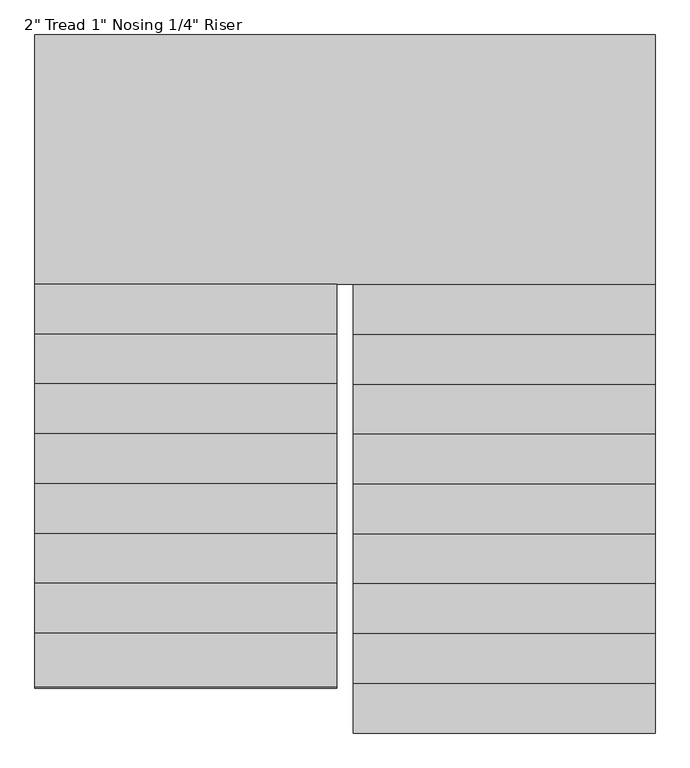
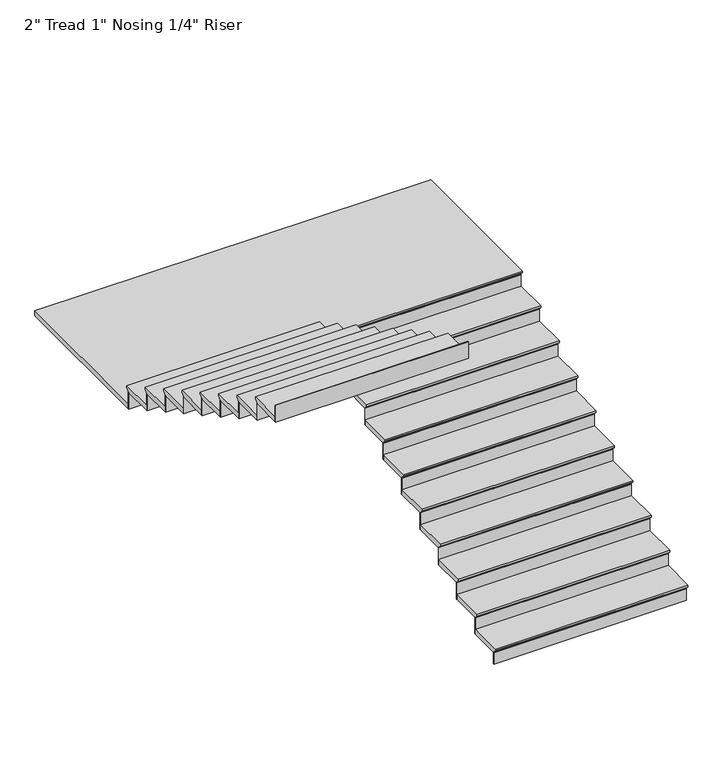
"""IFC4 building model written with IfcOpenShell, lengths in millimetres: stair flight geometry."""

from ifc_helpers import new_model, si_unit, origin, place, context, project, spatial, faceted_brep, source, transform, mapped, element, save


def stair_flight_059c6031(model_context):
    return source(origin(), model_context, "Body", "Brep", [
        faceted_brep([(7785.2813124, -8648.1976656, 4111.7921053), (7785.2813124, -8648.1976656, 4130.8421053), (5940.6255016, -8648.1976656, 4130.8421053), (5940.6255016, -8648.1976656, 4111.7921053), (7785.2813124, -8622.7976656, 4086.3921053), (5940.6255016, -8622.7976656, 4086.3921053), (7785.2813124, -8317.9976656, 4130.8421053), (5940.6255016, -8317.9976656, 4130.8421053), (5940.6255016, -8622.7976656, 4080.0421053), (5940.6255016, -8317.9976656, 4080.0421053), (7785.2813124, -8317.9976656, 4080.0421053), (7785.2813124, -8622.7976656, 4080.0421053)], [[[0, 1, 2, 3]], [[4, 0, 3, 5]], [[2, 1, 6, 7]], [[8, 9, 10, 11]], [[2, 7, 9, 8, 5, 3]], [[8, 11, 4, 5]], [[6, 1, 0, 4, 11, 10]], [[7, 6, 10, 9]]]),
        faceted_brep([(7785.2813124, -8622.7976656, 4080.0421053), (7785.2813124, -8622.7976656, 3962.4), (7785.2813124, -8616.4476656, 3962.4), (7785.2813124, -8616.4476656, 4080.0421053), (5940.6255016, -8622.7976656, 4080.0421053), (5940.6255016, -8616.4476656, 4080.0421053), (5940.6255016, -8616.4476656, 3962.4), (5940.6255016, -8622.7976656, 3962.4)], [[[0, 1, 2, 3]], [[4, 5, 6, 7]], [[1, 0, 4, 7]], [[2, 1, 7, 6]], [[3, 2, 6, 5]], [[0, 3, 5, 4]]]),
        faceted_brep([(7785.2813124, -8317.9976656, 4248.4842105), (7785.2813124, -8317.9976656, 4080.0421053), (7785.2813124, -8311.6476656, 4080.0421053), (7785.2813124, -8311.6476656, 4248.4842105), (5940.6255016, -8317.9976656, 4248.4842105), (5940.6255016, -8311.6476656, 4248.4842105), (5940.6255016, -8311.6476656, 4080.0421053), (5940.6255016, -8317.9976656, 4080.0421053)], [[[0, 1, 2, 3]], [[4, 5, 6, 7]], [[1, 0, 4, 7]], [[2, 1, 7, 6]], [[3, 2, 6, 5]], [[0, 3, 5, 4]]]),
        faceted_brep([(5940.6255016, -8343.3976656, 4299.2842105), (7785.2813124, -8343.3976656, 4299.2842105), (7785.2813124, -8013.1976656, 4299.2842105), (5940.6255016, -8013.1976656, 4299.2842105), (5940.6255016, -8317.9976656, 4248.4842105), (5940.6255016, -8013.1976656, 4248.4842105), (7785.2813124, -8013.1976656, 4248.4842105), (7785.2813124, -8317.9976656, 4248.4842105), (5940.6255016, -8317.9976656, 4254.8342105), (5940.6255016, -8343.3976656, 4280.2342105), (7785.2813124, -8317.9976656, 4254.8342105), (7785.2813124, -8343.3976656, 4280.2342105)], [[[0, 1, 2, 3]], [[4, 5, 6, 7]], [[0, 3, 5, 4, 8, 9]], [[4, 7, 10, 8]], [[2, 1, 11, 10, 7, 6]], [[3, 2, 6, 5]], [[11, 1, 0, 9]], [[10, 11, 9, 8]]]),
        faceted_brep([(7785.2813124, -8013.1976656, 4416.9263158), (7785.2813124, -8013.1976656, 4248.4842105), (7785.2813124, -8006.8476656, 4248.4842105), (7785.2813124, -8006.8476656, 4416.9263158), (5940.6255016, -8013.1976656, 4416.9263158), (5940.6255016, -8006.8476656, 4416.9263158), (5940.6255016, -8006.8476656, 4248.4842105), (5940.6255016, -8013.1976656, 4248.4842105)], [[[0, 1, 2, 3]], [[4, 5, 6, 7]], [[1, 0, 4, 7]], [[2, 1, 7, 6]], [[3, 2, 6, 5]], [[0, 3, 5, 4]]]),
        faceted_brep([(5940.6255016, -8038.5976656, 4467.7263158), (7785.2813124, -8038.5976656, 4467.7263158), (7785.2813124, -7708.3976656, 4467.7263158), (5940.6255016, -7708.3976656, 4467.7263158), (5940.6255016, -8013.1976656, 4416.9263158), (5940.6255016, -7708.3976656, 4416.9263158), (7785.2813124, -7708.3976656, 4416.9263158), (7785.2813124, -8013.1976656, 4416.9263158), (5940.6255016, -8013.1976656, 4423.2763158), (5940.6255016, -8038.5976656, 4448.6763158), (7785.2813124, -8013.1976656, 4423.2763158), (7785.2813124, -8038.5976656, 4448.6763158)], [[[0, 1, 2, 3]], [[4, 5, 6, 7]], [[0, 3, 5, 4, 8, 9]], [[4, 7, 10, 8]], [[2, 1, 11, 10, 7, 6]], [[3, 2, 6, 5]], [[11, 1, 0, 9]], [[10, 11, 9, 8]]]),
        faceted_brep([(7785.2813124, -7708.3976656, 4585.3684211), (7785.2813124, -7708.3976656, 4416.9263158), (7785.2813124, -7702.0476656, 4416.9263158), (7785.2813124, -7702.0476656, 4585.3684211), (5940.6255016, -7708.3976656, 4585.3684211), (5940.6255016, -7702.0476656, 4585.3684211), (5940.6255016, -7702.0476656, 4416.9263158), (5940.6255016, -7708.3976656, 4416.9263158)], [[[0, 1, 2, 3]], [[4, 5, 6, 7]], [[1, 0, 4, 7]], [[2, 1, 7, 6]], [[3, 2, 6, 5]], [[0, 3, 5, 4]]]),
        faceted_brep([(5940.6255016, -7733.7976656, 4636.1684211), (7785.2813124, -7733.7976656, 4636.1684211), (7785.2813124, -7403.5976656, 4636.1684211), (5940.6255016, -7403.5976656, 4636.1684211), (5940.6255016, -7708.3976656, 4585.3684211), (5940.6255016, -7403.5976656, 4585.3684211), (7785.2813124, -7403.5976656, 4585.3684211), (7785.2813124, -7708.3976656, 4585.3684211), (5940.6255016, -7708.3976656, 4591.7184211), (5940.6255016, -7733.7976656, 4617.1184211), (7785.2813124, -7708.3976656, 4591.7184211), (7785.2813124, -7733.7976656, 4617.1184211)], [[[0, 1, 2, 3]], [[4, 5, 6, 7]], [[0, 3, 5, 4, 8, 9]], [[4, 7, 10, 8]], [[2, 1, 11, 10, 7, 6]], [[3, 2, 6, 5]], [[11, 1, 0, 9]], [[10, 11, 9, 8]]]),
        faceted_brep([(7785.2813124, -7403.5976656, 4753.8105263), (7785.2813124, -7403.5976656, 4585.3684211), (7785.2813124, -7397.2476656, 4585.3684211), (7785.2813124, -7397.2476656, 4753.8105263), (5940.6255016, -7403.5976656, 4753.8105263), (5940.6255016, -7397.2476656, 4753.8105263), (5940.6255016, -7397.2476656, 4585.3684211), (5940.6255016, -7403.5976656, 4585.3684211)], [[[0, 1, 2, 3]], [[4, 5, 6, 7]], [[1, 0, 4, 7]], [[2, 1, 7, 6]], [[3, 2, 6, 5]], [[0, 3, 5, 4]]]),
        faceted_brep([(5940.6255016, -7428.9976656, 4804.6105263), (7785.2813124, -7428.9976656, 4804.6105263), (7785.2813124, -7098.7976656, 4804.6105263), (5940.6255016, -7098.7976656, 4804.6105263), (5940.6255016, -7403.5976656, 4753.8105263), (5940.6255016, -7098.7976656, 4753.8105263), (7785.2813124, -7098.7976656, 4753.8105263), (7785.2813124, -7403.5976656, 4753.8105263), (5940.6255016, -7403.5976656, 4760.1605263), (5940.6255016, -7428.9976656, 4785.5605263), (7785.2813124, -7403.5976656, 4760.1605263), (7785.2813124, -7428.9976656, 4785.5605263)], [[[0, 1, 2, 3]], [[4, 5, 6, 7]], [[0, 3, 5, 4, 8, 9]], [[4, 7, 10, 8]], [[2, 1, 11, 10, 7, 6]], [[3, 2, 6, 5]], [[11, 1, 0, 9]], [[10, 11, 9, 8]]]),
        faceted_brep([(7785.2813124, -7098.7976656, 4922.2526316), (7785.2813124, -7098.7976656, 4753.8105263), (7785.2813124, -7092.4476656, 4753.8105263), (7785.2813124, -7092.4476656, 4922.2526316), (5940.6255016, -7098.7976656, 4922.2526316), (5940.6255016, -7092.4476656, 4922.2526316), (5940.6255016, -7092.4476656, 4753.8105263), (5940.6255016, -7098.7976656, 4753.8105263)], [[[0, 1, 2, 3]], [[4, 5, 6, 7]], [[1, 0, 4, 7]], [[2, 1, 7, 6]], [[3, 2, 6, 5]], [[0, 3, 5, 4]]]),
        faceted_brep([(5940.6255016, -7124.1976656, 4973.0526316), (7785.2813124, -7124.1976656, 4973.0526316), (7785.2813124, -6793.9976656, 4973.0526316), (5940.6255016, -6793.9976656, 4973.0526316), (5940.6255016, -7098.7976656, 4922.2526316), (5940.6255016, -6793.9976656, 4922.2526316), (7785.2813124, -6793.9976656, 4922.2526316), (7785.2813124, -7098.7976656, 4922.2526316), (5940.6255016, -7098.7976656, 4928.6026316), (5940.6255016, -7124.1976656, 4954.0026316), (7785.2813124, -7098.7976656, 4928.6026316), (7785.2813124, -7124.1976656, 4954.0026316)], [[[0, 1, 2, 3]], [[4, 5, 6, 7]], [[0, 3, 5, 4, 8, 9]], [[4, 7, 10, 8]], [[2, 1, 11, 10, 7, 6]], [[3, 2, 6, 5]], [[11, 1, 0, 9]], [[10, 11, 9, 8]]]),
        faceted_brep([(7785.2813124, -6793.9976656, 5090.6947368), (7785.2813124, -6793.9976656, 4922.2526316), (7785.2813124, -6787.6476656, 4922.2526316), (7785.2813124, -6787.6476656, 5090.6947368), (5940.6255016, -6793.9976656, 5090.6947368), (5940.6255016, -6787.6476656, 5090.6947368), (5940.6255016, -6787.6476656, 4922.2526316), (5940.6255016, -6793.9976656, 4922.2526316)], [[[0, 1, 2, 3]], [[4, 5, 6, 7]], [[1, 0, 4, 7]], [[2, 1, 7, 6]], [[3, 2, 6, 5]], [[0, 3, 5, 4]]]),
        faceted_brep([(5940.6255016, -6819.3976656, 5141.4947368), (7785.2813124, -6819.3976656, 5141.4947368), (7785.2813124, -6489.1976656, 5141.4947368), (5940.6255016, -6489.1976656, 5141.4947368), (5940.6255016, -6793.9976656, 5090.6947368), (5940.6255016, -6489.1976656, 5090.6947368), (7785.2813124, -6489.1976656, 5090.6947368), (7785.2813124, -6793.9976656, 5090.6947368), (5940.6255016, -6793.9976656, 5097.0447368), (5940.6255016, -6819.3976656, 5122.4447368), (7785.2813124, -6793.9976656, 5097.0447368), (7785.2813124, -6819.3976656, 5122.4447368)], [[[0, 1, 2, 3]], [[4, 5, 6, 7]], [[0, 3, 5, 4, 8, 9]], [[4, 7, 10, 8]], [[2, 1, 11, 10, 7, 6]], [[3, 2, 6, 5]], [[11, 1, 0, 9]], [[10, 11, 9, 8]]]),
        faceted_brep([(7785.2813124, -6489.1976656, 5259.1368421), (7785.2813124, -6489.1976656, 5090.6947368), (7785.2813124, -6482.8476656, 5090.6947368), (7785.2813124, -6482.8476656, 5259.1368421), (5940.6255016, -6489.1976656, 5259.1368421), (5940.6255016, -6482.8476656, 5259.1368421), (5940.6255016, -6482.8476656, 5090.6947368), (5940.6255016, -6489.1976656, 5090.6947368)], [[[0, 1, 2, 3]], [[4, 5, 6, 7]], [[1, 0, 4, 7]], [[2, 1, 7, 6]], [[3, 2, 6, 5]], [[0, 3, 5, 4]]]),
        faceted_brep([(5940.6255016, -6514.5976656, 5309.9368421), (7785.2813124, -6514.5976656, 5309.9368421), (7785.2813124, -6184.3976656, 5309.9368421), (5940.6255016, -6184.3976656, 5309.9368421), (5940.6255016, -6489.1976656, 5259.1368421), (5940.6255016, -6184.3976656, 5259.1368421), (7785.2813124, -6184.3976656, 5259.1368421), (7785.2813124, -6489.1976656, 5259.1368421), (5940.6255016, -6489.1976656, 5265.4868421), (5940.6255016, -6514.5976656, 5290.8868421), (7785.2813124, -6489.1976656, 5265.4868421), (7785.2813124, -6514.5976656, 5290.8868421)], [[[0, 1, 2, 3]], [[4, 5, 6, 7]], [[0, 3, 5, 4, 8, 9]], [[4, 7, 10, 8]], [[2, 1, 11, 10, 7, 6]], [[3, 2, 6, 5]], [[11, 1, 0, 9]], [[10, 11, 9, 8]]]),
        faceted_brep([(7785.2813124, -5879.5976656, 5596.0210526), (7785.2813124, -5879.5976656, 5427.5789474), (7785.2813124, -5873.2476656, 5427.5789474), (7785.2813124, -5873.2476656, 5596.0210526), (5940.6255016, -5879.5976656, 5596.0210526), (5940.6255016, -5873.2476656, 5596.0210526), (5940.6255016, -5873.2476656, 5427.5789474), (5940.6255016, -5879.5976656, 5427.5789474)], [[[0, 1, 2, 3]], [[4, 5, 6, 7]], [[1, 0, 4, 7]], [[2, 1, 7, 6]], [[3, 2, 6, 5]], [[0, 3, 5, 4]]]),
        faceted_brep([(5839.0255016, -5930.3976656, 5646.8210526), (5839.0255016, -5904.9976656, 5646.8210526), (7785.2813124, -5904.9976656, 5646.8210526), (7785.2813124, -4380.9976656, 5646.8210526), (3994.3696908, -4380.9976656, 5646.8210526), (3994.3696908, -5930.3976656, 5646.8210526), (5839.0255016, -5904.9976656, 5596.0210526), (5839.0255016, -5930.3976656, 5596.0210526), (3994.3696908, -5930.3976656, 5596.0210526), (3994.3696908, -4380.9976656, 5596.0210526), (7785.2813124, -4380.9976656, 5596.0210526), (7785.2813124, -5879.5976656, 5596.0210526), (5940.6255016, -5879.5976656, 5596.0210526), (5940.6255016, -5904.9976656, 5596.0210526), (7785.2813124, -5879.5976656, 5602.3710526), (5940.6255016, -5879.5976656, 5602.3710526), (7785.2813124, -5904.9976656, 5627.7710526), (5940.6255016, -5904.9976656, 5627.7710526)], [[[0, 1, 2, 3, 4, 5]], [[6, 7, 8, 9, 10, 11, 12, 13]], [[1, 0, 7, 6]], [[12, 11, 14, 15]], [[3, 2, 16, 14, 11, 10]], [[0, 5, 8, 7]], [[14, 16, 17, 15]], [[2, 1, 6, 13, 17, 16]], [[13, 12, 15, 17]], [[4, 3, 10, 9]], [[5, 4, 9, 8]]]),
        faceted_brep([(3994.3696908, -8368.7976656, 7112.0), (3994.3696908, -8368.7976656, 6943.5578947), (3994.3696908, -8375.1476656, 6943.5578947), (3994.3696908, -8375.1476656, 7112.0), (5839.0255016, -8368.7976656, 7112.0), (5839.0255016, -8375.1476656, 7112.0), (5839.0255016, -8375.1476656, 6943.5578947), (5839.0255016, -8368.7976656, 6943.5578947)], [[[0, 1, 2, 3]], [[4, 5, 6, 7]], [[1, 0, 4, 7]], [[2, 1, 7, 6]], [[3, 2, 6, 5]], [[0, 3, 5, 4]]]),
        faceted_brep([(7785.2813124, -6184.3976656, 5427.5789474), (7785.2813124, -6184.3976656, 5259.1368421), (7785.2813124, -6178.0476656, 5259.1368421), (7785.2813124, -6178.0476656, 5427.5789474), (5940.6255016, -6184.3976656, 5427.5789474), (5940.6255016, -6178.0476656, 5427.5789474), (5940.6255016, -6178.0476656, 5259.1368421), (5940.6255016, -6184.3976656, 5259.1368421)], [[[0, 1, 2, 3]], [[4, 5, 6, 7]], [[1, 0, 4, 7]], [[2, 1, 7, 6]], [[3, 2, 6, 5]], [[0, 3, 5, 4]]]),
        faceted_brep([(5940.6255016, -6209.7976656, 5478.3789474), (7785.2813124, -6209.7976656, 5478.3789474), (7785.2813124, -5879.5976656, 5478.3789474), (5940.6255016, -5879.5976656, 5478.3789474), (5940.6255016, -6184.3976656, 5427.5789474), (5940.6255016, -5879.5976656, 5427.5789474), (7785.2813124, -5879.5976656, 5427.5789474), (7785.2813124, -6184.3976656, 5427.5789474), (5940.6255016, -6184.3976656, 5433.9289474), (5940.6255016, -6209.7976656, 5459.3289474), (7785.2813124, -6184.3976656, 5433.9289474), (7785.2813124, -6209.7976656, 5459.3289474)], [[[0, 1, 2, 3]], [[4, 5, 6, 7]], [[0, 3, 5, 4, 8, 9]], [[4, 7, 10, 8]], [[2, 1, 11, 10, 7, 6]], [[3, 2, 6, 5]], [[11, 1, 0, 9]], [[10, 11, 9, 8]]]),
        faceted_brep([(3994.3696908, -5930.3976656, 5764.4631579), (3994.3696908, -5930.3976656, 5596.0210526), (3994.3696908, -5936.7476656, 5596.0210526), (3994.3696908, -5936.7476656, 5764.4631579), (5839.0255016, -5930.3976656, 5764.4631579), (5839.0255016, -5936.7476656, 5764.4631579), (5839.0255016, -5936.7476656, 5596.0210526), (5839.0255016, -5930.3976656, 5596.0210526)], [[[0, 1, 2, 3]], [[4, 5, 6, 7]], [[1, 0, 4, 7]], [[2, 1, 7, 6]], [[3, 2, 6, 5]], [[0, 3, 5, 4]]]),
        faceted_brep([(5839.0255016, -5904.9976656, 5815.2631579), (3994.3696908, -5904.9976656, 5815.2631579), (3994.3696908, -6235.1976656, 5815.2631579), (5839.0255016, -6235.1976656, 5815.2631579), (5839.0255016, -5930.3976656, 5764.4631579), (5839.0255016, -6235.1976656, 5764.4631579), (3994.3696908, -6235.1976656, 5764.4631579), (3994.3696908, -5930.3976656, 5764.4631579), (5839.0255016, -5930.3976656, 5770.8131579), (5839.0255016, -5904.9976656, 5796.2131579), (3994.3696908, -5930.3976656, 5770.8131579), (3994.3696908, -5904.9976656, 5796.2131579)], [[[0, 1, 2, 3]], [[4, 5, 6, 7]], [[0, 3, 5, 4, 8, 9]], [[4, 7, 10, 8]], [[2, 1, 11, 10, 7, 6]], [[3, 2, 6, 5]], [[11, 1, 0, 9]], [[10, 11, 9, 8]]]),
        faceted_brep([(3994.3696908, -6235.1976656, 5932.9052632), (3994.3696908, -6235.1976656, 5764.4631579), (3994.3696908, -6241.5476656, 5764.4631579), (3994.3696908, -6241.5476656, 5932.9052632), (5839.0255016, -6235.1976656, 5932.9052632), (5839.0255016, -6241.5476656, 5932.9052632), (5839.0255016, -6241.5476656, 5764.4631579), (5839.0255016, -6235.1976656, 5764.4631579)], [[[0, 1, 2, 3]], [[4, 5, 6, 7]], [[1, 0, 4, 7]], [[2, 1, 7, 6]], [[3, 2, 6, 5]], [[0, 3, 5, 4]]]),
        faceted_brep([(5839.0255016, -6209.7976656, 5983.7052632), (3994.3696908, -6209.7976656, 5983.7052632), (3994.3696908, -6539.9976656, 5983.7052632), (5839.0255016, -6539.9976656, 5983.7052632), (5839.0255016, -6235.1976656, 5932.9052632), (5839.0255016, -6539.9976656, 5932.9052632), (3994.3696908, -6539.9976656, 5932.9052632), (3994.3696908, -6235.1976656, 5932.9052632), (5839.0255016, -6235.1976656, 5939.2552632), (5839.0255016, -6209.7976656, 5964.6552632), (3994.3696908, -6235.1976656, 5939.2552632), (3994.3696908, -6209.7976656, 5964.6552632)], [[[0, 1, 2, 3]], [[4, 5, 6, 7]], [[0, 3, 5, 4, 8, 9]], [[4, 7, 10, 8]], [[2, 1, 11, 10, 7, 6]], [[3, 2, 6, 5]], [[11, 1, 0, 9]], [[10, 11, 9, 8]]]),
        faceted_brep([(3994.3696908, -6539.9976656, 6101.3473684), (3994.3696908, -6539.9976656, 5932.9052632), (3994.3696908, -6546.3476656, 5932.9052632), (3994.3696908, -6546.3476656, 6101.3473684), (5839.0255016, -6539.9976656, 6101.3473684), (5839.0255016, -6546.3476656, 6101.3473684), (5839.0255016, -6546.3476656, 5932.9052632), (5839.0255016, -6539.9976656, 5932.9052632)], [[[0, 1, 2, 3]], [[4, 5, 6, 7]], [[1, 0, 4, 7]], [[2, 1, 7, 6]], [[3, 2, 6, 5]], [[0, 3, 5, 4]]]),
        faceted_brep([(5839.0255016, -6514.5976656, 6152.1473684), (3994.3696908, -6514.5976656, 6152.1473684), (3994.3696908, -6844.7976656, 6152.1473684), (5839.0255016, -6844.7976656, 6152.1473684), (5839.0255016, -6539.9976656, 6101.3473684), (5839.0255016, -6844.7976656, 6101.3473684), (3994.3696908, -6844.7976656, 6101.3473684), (3994.3696908, -6539.9976656, 6101.3473684), (5839.0255016, -6539.9976656, 6107.6973684), (5839.0255016, -6514.5976656, 6133.0973684), (3994.3696908, -6539.9976656, 6107.6973684), (3994.3696908, -6514.5976656, 6133.0973684)], [[[0, 1, 2, 3]], [[4, 5, 6, 7]], [[0, 3, 5, 4, 8, 9]], [[4, 7, 10, 8]], [[2, 1, 11, 10, 7, 6]], [[3, 2, 6, 5]], [[11, 1, 0, 9]], [[10, 11, 9, 8]]]),
        faceted_brep([(3994.3696908, -6844.7976656, 6269.7894737), (3994.3696908, -6844.7976656, 6101.3473684), (3994.3696908, -6851.1476656, 6101.3473684), (3994.3696908, -6851.1476656, 6269.7894737), (5839.0255016, -6844.7976656, 6269.7894737), (5839.0255016, -6851.1476656, 6269.7894737), (5839.0255016, -6851.1476656, 6101.3473684), (5839.0255016, -6844.7976656, 6101.3473684)], [[[0, 1, 2, 3]], [[4, 5, 6, 7]], [[1, 0, 4, 7]], [[2, 1, 7, 6]], [[3, 2, 6, 5]], [[0, 3, 5, 4]]]),
        faceted_brep([(5839.0255016, -6819.3976656, 6320.5894737), (3994.3696908, -6819.3976656, 6320.5894737), (3994.3696908, -7149.5976656, 6320.5894737), (5839.0255016, -7149.5976656, 6320.5894737), (5839.0255016, -6844.7976656, 6269.7894737), (5839.0255016, -7149.5976656, 6269.7894737), (3994.3696908, -7149.5976656, 6269.7894737), (3994.3696908, -6844.7976656, 6269.7894737), (5839.0255016, -6844.7976656, 6276.1394737), (5839.0255016, -6819.3976656, 6301.5394737), (3994.3696908, -6844.7976656, 6276.1394737), (3994.3696908, -6819.3976656, 6301.5394737)], [[[0, 1, 2, 3]], [[4, 5, 6, 7]], [[0, 3, 5, 4, 8, 9]], [[4, 7, 10, 8]], [[2, 1, 11, 10, 7, 6]], [[3, 2, 6, 5]], [[11, 1, 0, 9]], [[10, 11, 9, 8]]]),
        faceted_brep([(3994.3696908, -7149.5976656, 6438.2315789), (3994.3696908, -7149.5976656, 6269.7894737), (3994.3696908, -7155.9476656, 6269.7894737), (3994.3696908, -7155.9476656, 6438.2315789), (5839.0255016, -7149.5976656, 6438.2315789), (5839.0255016, -7155.9476656, 6438.2315789), (5839.0255016, -7155.9476656, 6269.7894737), (5839.0255016, -7149.5976656, 6269.7894737)], [[[0, 1, 2, 3]], [[4, 5, 6, 7]], [[1, 0, 4, 7]], [[2, 1, 7, 6]], [[3, 2, 6, 5]], [[0, 3, 5, 4]]]),
        faceted_brep([(5839.0255016, -7124.1976656, 6489.0315789), (3994.3696908, -7124.1976656, 6489.0315789), (3994.3696908, -7454.3976656, 6489.0315789), (5839.0255016, -7454.3976656, 6489.0315789), (5839.0255016, -7149.5976656, 6438.2315789), (5839.0255016, -7454.3976656, 6438.2315789), (3994.3696908, -7454.3976656, 6438.2315789), (3994.3696908, -7149.5976656, 6438.2315789), (5839.0255016, -7149.5976656, 6444.5815789), (5839.0255016, -7124.1976656, 6469.9815789), (3994.3696908, -7149.5976656, 6444.5815789), (3994.3696908, -7124.1976656, 6469.9815789)], [[[0, 1, 2, 3]], [[4, 5, 6, 7]], [[0, 3, 5, 4, 8, 9]], [[4, 7, 10, 8]], [[2, 1, 11, 10, 7, 6]], [[3, 2, 6, 5]], [[11, 1, 0, 9]], [[10, 11, 9, 8]]]),
        faceted_brep([(3994.3696908, -7454.3976656, 6606.6736842), (3994.3696908, -7454.3976656, 6438.2315789), (3994.3696908, -7460.7476656, 6438.2315789), (3994.3696908, -7460.7476656, 6606.6736842), (5839.0255016, -7454.3976656, 6606.6736842), (5839.0255016, -7460.7476656, 6606.6736842), (5839.0255016, -7460.7476656, 6438.2315789), (5839.0255016, -7454.3976656, 6438.2315789)], [[[0, 1, 2, 3]], [[4, 5, 6, 7]], [[1, 0, 4, 7]], [[2, 1, 7, 6]], [[3, 2, 6, 5]], [[0, 3, 5, 4]]]),
        faceted_brep([(5839.0255016, -7428.9976656, 6657.4736842), (3994.3696908, -7428.9976656, 6657.4736842), (3994.3696908, -7759.1976656, 6657.4736842), (5839.0255016, -7759.1976656, 6657.4736842), (5839.0255016, -7454.3976656, 6606.6736842), (5839.0255016, -7759.1976656, 6606.6736842), (3994.3696908, -7759.1976656, 6606.6736842), (3994.3696908, -7454.3976656, 6606.6736842), (5839.0255016, -7454.3976656, 6613.0236842), (5839.0255016, -7428.9976656, 6638.4236842), (3994.3696908, -7454.3976656, 6613.0236842), (3994.3696908, -7428.9976656, 6638.4236842)], [[[0, 1, 2, 3]], [[4, 5, 6, 7]], [[0, 3, 5, 4, 8, 9]], [[4, 7, 10, 8]], [[2, 1, 11, 10, 7, 6]], [[3, 2, 6, 5]], [[11, 1, 0, 9]], [[10, 11, 9, 8]]]),
        faceted_brep([(3994.3696908, -7759.1976656, 6775.1157895), (3994.3696908, -7759.1976656, 6606.6736842), (3994.3696908, -7765.5476656, 6606.6736842), (3994.3696908, -7765.5476656, 6775.1157895), (5839.0255016, -7759.1976656, 6775.1157895), (5839.0255016, -7765.5476656, 6775.1157895), (5839.0255016, -7765.5476656, 6606.6736842), (5839.0255016, -7759.1976656, 6606.6736842)], [[[0, 1, 2, 3]], [[4, 5, 6, 7]], [[1, 0, 4, 7]], [[2, 1, 7, 6]], [[3, 2, 6, 5]], [[0, 3, 5, 4]]]),
        faceted_brep([(5839.0255016, -7733.7976656, 6825.9157895), (3994.3696908, -7733.7976656, 6825.9157895), (3994.3696908, -8063.9976656, 6825.9157895), (5839.0255016, -8063.9976656, 6825.9157895), (5839.0255016, -7759.1976656, 6775.1157895), (5839.0255016, -8063.9976656, 6775.1157895), (3994.3696908, -8063.9976656, 6775.1157895), (3994.3696908, -7759.1976656, 6775.1157895), (5839.0255016, -7759.1976656, 6781.4657895), (5839.0255016, -7733.7976656, 6806.8657895), (3994.3696908, -7759.1976656, 6781.4657895), (3994.3696908, -7733.7976656, 6806.8657895)], [[[0, 1, 2, 3]], [[4, 5, 6, 7]], [[0, 3, 5, 4, 8, 9]], [[4, 7, 10, 8]], [[2, 1, 11, 10, 7, 6]], [[3, 2, 6, 5]], [[11, 1, 0, 9]], [[10, 11, 9, 8]]]),
        faceted_brep([(3994.3696908, -8063.9976656, 6943.5578947), (3994.3696908, -8063.9976656, 6775.1157895), (3994.3696908, -8070.3476656, 6775.1157895), (3994.3696908, -8070.3476656, 6943.5578947), (5839.0255016, -8063.9976656, 6943.5578947), (5839.0255016, -8070.3476656, 6943.5578947), (5839.0255016, -8070.3476656, 6775.1157895), (5839.0255016, -8063.9976656, 6775.1157895)], [[[0, 1, 2, 3]], [[4, 5, 6, 7]], [[1, 0, 4, 7]], [[2, 1, 7, 6]], [[3, 2, 6, 5]], [[0, 3, 5, 4]]]),
        faceted_brep([(5839.0255016, -8038.5976656, 6994.3578947), (3994.3696908, -8038.5976656, 6994.3578947), (3994.3696908, -8368.7976656, 6994.3578947), (5839.0255016, -8368.7976656, 6994.3578947), (5839.0255016, -8063.9976656, 6943.5578947), (5839.0255016, -8368.7976656, 6943.5578947), (3994.3696908, -8368.7976656, 6943.5578947), (3994.3696908, -8063.9976656, 6943.5578947), (5839.0255016, -8063.9976656, 6949.9078947), (5839.0255016, -8038.5976656, 6975.3078947), (3994.3696908, -8063.9976656, 6949.9078947), (3994.3696908, -8038.5976656, 6975.3078947)], [[[0, 1, 2, 3]], [[4, 5, 6, 7]], [[0, 3, 5, 4, 8, 9]], [[4, 7, 10, 8]], [[2, 1, 11, 10, 7, 6]], [[3, 2, 6, 5]], [[11, 1, 0, 9]], [[10, 11, 9, 8]]]),
    ])


if __name__ == "__main__":
    model = new_model("IFC4")
    model_context = context("Model", 3, world=origin())
    ifc_project = project(units=[si_unit("LENGTHUNIT", "METRE", prefix="MILLI")], contexts=[model_context])
    site = spatial("IfcSite", under=ifc_project)
    building = spatial("IfcBuilding", under=site)
    placement = place(None, origin())
    stair_flight_shape = stair_flight_059c6031(model_context)
    element("IfcStairFlight", 1, ObjectType="2\" Tread 1\" Nosing 1/4\" Riser", at=placement, inside=building, context=model_context, shape_type="MappedRepresentation", body=[
        mapped(stair_flight_shape, transform((0.0, 0.0, 0.0), x_axis=(1.0, 0.0, 0.0), y_axis=(0.0, 1.0, 0.0), z_axis=(0.0, 0.0, 1.0))),
    ])
    save(model, "model.ifc")
